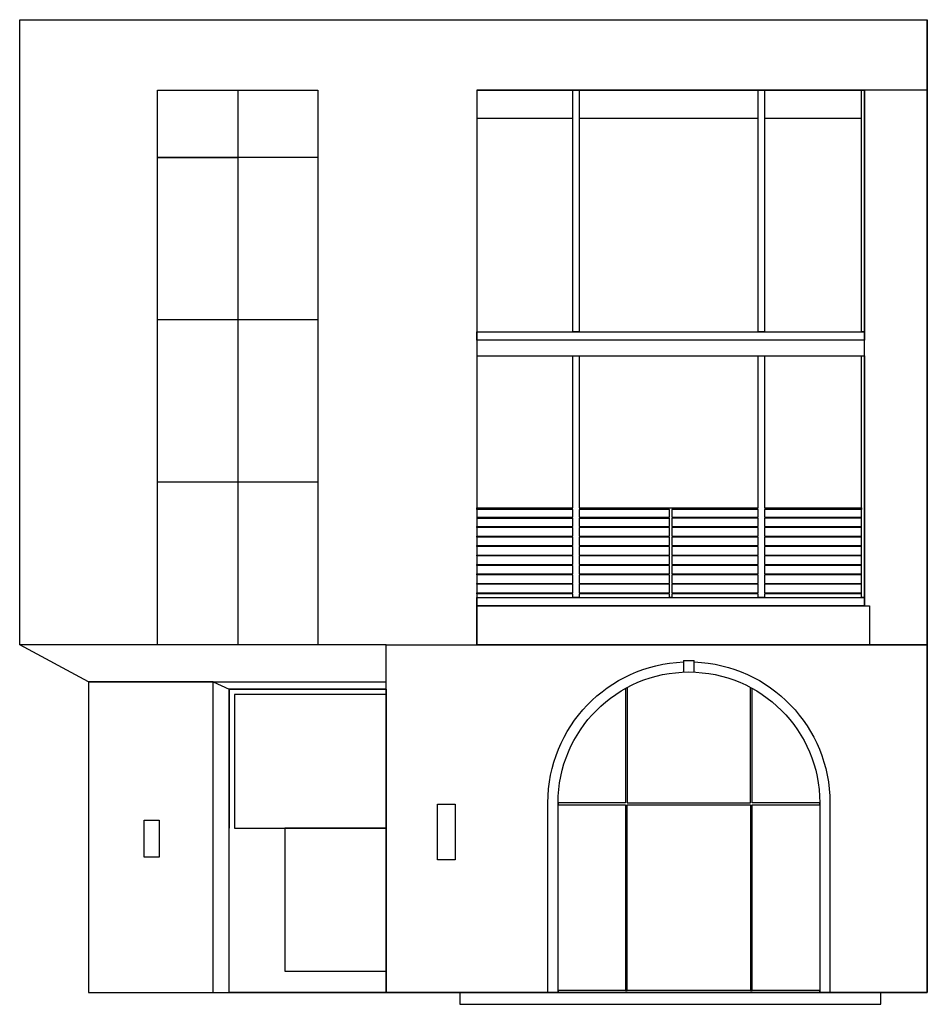
# Model space of a CAD drawing. Units: feet. Extents: x 2368 to 3224, y 836 to 1229.
# Tile 9 of 9: x 2873 to 3224, y 849 to 1229. Entities that reach past the tile are written whole.
import ezdxf

# ---------------------------------------------------------------- set-up
doc = ezdxf.new("R2010")
doc.units = ezdxf.units.FT
doc.layers.add('A-ELEV', color=7, linetype='Continuous', lineweight=25)

msp = doc.modelspace()

# ---------------------------------------------------------------- linework, layer by layer
at = {"layer": 'A-ELEV'}
for p, q in [((2872.69, 987.86), (2872.69, 1229.35)), ((3223.55, 853.51), (3223.55, 1229.35)), ((2956.97, 1202.15), (2956.97, 987.86)), ((3049.37, 1202.15), (3199.32, 1202.15)), ((3086.5, 1191.22), (3049.37, 1191.22)), ((3158.11, 1191.22), (3088.99, 1191.22)), ((3198.12, 1191.22), (3160.6, 1191.22)), ((2987.91, 1176.09), (2926.02, 1176.09)), ((3199.32, 1105.51), (3049.37, 1105.51)), ((3049.37, 1099.51), (3199.32, 1099.51)), ((3049.37, 1037.14), (3086.5, 1037.14)), ((3049.37, 1036.77), (3086.5, 1036.77)), ((3088.99, 1037.14), (3123.88, 1037.14)), ((3088.99, 1036.77), (3123.88, 1036.77)), ((3014.41, 987.86), (2872.69, 987.86)), ((2899.3, 973.51), (2872.69, 987.86)), ((2899.3, 973.51), (3014.41, 973.51)), ((2947.43, 973.51), (2953.69, 970.69)), ((2899.3, 853.51), (3223.55, 853.51))]:
    msp.add_line(p, q, dxfattribs=at)
for points in [[(2872.69, 1229.35), (3223.55, 1229.35), (3223.55, 1202.15), (3049.37, 1202.15)], [(3223.55, 1229.35), (3223.55, 987.86), (3199.32, 987.86)], [(3049.37, 1202.15), (3049.37, 987.86)], [(3199.32, 1002.87), (3199.32, 1202.15)], [(2987.91, 1113.35), (2926.02, 1113.35), (2926.02, 1176.09), (2956.97, 1176.09)], [(2987.91, 1113.35), (2987.91, 1050.6), (2926.02, 1050.6)], [(3086.5, 1040.78), (3086.5, 1099.51), (3088.99, 1099.51), (3088.99, 1040.78)], [(3158.11, 1040.78), (3158.11, 1099.51), (3160.6, 1099.51), (3160.6, 1040.78)], [(2962.72, 987.86), (2926.02, 987.86), (2926.02, 1050.6)], [(3086.5, 1040.06), (3049.37, 1040.06), (3049.37, 1040.78), (3086.5, 1040.78)], [(3086.5, 1037.14), (3086.5, 1040.06)], [(3088.99, 1040.78), (3158.11, 1040.78)], [(3088.99, 1040.06), (3088.99, 1037.14)], [(3123.88, 1040.06), (3088.99, 1040.06)], [(3123.88, 1037.14), (3123.88, 1040.06)], [(3124.82, 1040.06), (3124.82, 1037.14)], [(3158.11, 1040.06), (3124.82, 1040.06)], [(3158.11, 1037.14), (3158.11, 1040.06)], [(3160.6, 1040.78), (3198.12, 1040.78), (3198.12, 1040.06), (3160.6, 1040.06)], [(3160.6, 1040.06), (3160.6, 1037.14)], [(3086.5, 1033.48), (3086.5, 1036.77)], [(3088.99, 1036.77), (3088.99, 1033.48)], [(3123.88, 1033.48), (3123.88, 1036.77)], [(3124.82, 1037.14), (3158.11, 1037.14)], [(3124.82, 1036.77), (3124.82, 1033.48)], [(3158.11, 1036.77), (3124.82, 1036.77)], [(3158.11, 1033.48), (3158.11, 1036.77)], [(3160.6, 1037.14), (3198.12, 1037.14)], [(3198.12, 1036.77), (3160.6, 1036.77)], [(3160.6, 1036.77), (3160.6, 1033.48)], [(3199.32, 1037.14), (3199.32, 1036.77)], [(3086.5, 1033.11), (3049.37, 1033.11), (3049.37, 1033.48), (3086.5, 1033.48)], [(3086.5, 1029.83), (3086.5, 1033.11)], [(3088.99, 1033.48), (3123.88, 1033.48)], [(3088.99, 1033.11), (3088.99, 1029.83)], [(3123.88, 1033.11), (3088.99, 1033.11)], [(3123.88, 1029.83), (3123.88, 1033.11)], [(3124.82, 1033.48), (3158.11, 1033.48)], [(3124.82, 1033.11), (3124.82, 1029.83)], [(3158.11, 1033.11), (3124.82, 1033.11)], [(3158.11, 1029.83), (3158.11, 1033.11)], [(3160.6, 1033.48), (3198.12, 1033.48)], [(3198.12, 1033.11), (3160.6, 1033.11)], [(3160.6, 1033.11), (3160.6, 1029.83)], [(3199.32, 1033.48), (3199.32, 1033.11)], [(3086.5, 1029.46), (3049.37, 1029.46), (3049.37, 1029.83), (3086.5, 1029.83)], [(3086.5, 1026.18), (3086.5, 1029.46)], [(3088.99, 1029.83), (3123.88, 1029.83)], [(3088.99, 1029.46), (3088.99, 1026.18)], [(3123.88, 1029.46), (3088.99, 1029.46)], [(3123.88, 1026.18), (3123.88, 1029.46)], [(3124.82, 1029.83), (3158.11, 1029.83)], [(3124.82, 1029.46), (3124.82, 1026.18)], [(3158.11, 1029.46), (3124.82, 1029.46)], [(3158.11, 1026.18), (3158.11, 1029.46)], [(3160.6, 1029.83), (3198.12, 1029.83)], [(3198.12, 1029.46), (3160.6, 1029.46)], [(3160.6, 1029.46), (3160.6, 1026.18)], [(3199.32, 1029.83), (3199.32, 1029.46)], [(3086.5, 1025.81), (3049.37, 1025.81), (3049.37, 1026.18), (3086.5, 1026.18)], [(3086.5, 1022.52), (3086.5, 1025.81)], [(3088.99, 1026.18), (3123.88, 1026.18)], [(3088.99, 1025.81), (3088.99, 1022.52)], [(3123.88, 1025.81), (3088.99, 1025.81)], [(3123.88, 1022.52), (3123.88, 1025.81)], [(3124.82, 1026.18), (3158.11, 1026.18)], [(3124.82, 1025.81), (3124.82, 1022.52)], [(3158.11, 1025.81), (3124.82, 1025.81)], [(3158.11, 1022.52), (3158.11, 1025.81)], [(3160.6, 1026.18), (3198.12, 1026.18)], [(3198.12, 1025.81), (3160.6, 1025.81)], [(3160.6, 1025.81), (3160.6, 1022.52)], [(3199.32, 1026.18), (3199.32, 1025.81)], [(3086.5, 1022.15), (3049.37, 1022.15), (3049.37, 1022.52), (3086.5, 1022.52)], [(3086.5, 1018.87), (3086.5, 1022.15)], [(3088.99, 1022.52), (3123.88, 1022.52)], [(3088.99, 1022.15), (3088.99, 1018.87)], [(3123.88, 1022.15), (3088.99, 1022.15)], [(3123.88, 1018.87), (3123.88, 1022.15)], [(3124.82, 1022.52), (3158.11, 1022.52)], [(3124.82, 1022.15), (3124.82, 1018.87)], [(3158.11, 1022.15), (3124.82, 1022.15)], [(3158.11, 1018.87), (3158.11, 1022.15)], [(3160.6, 1022.52), (3198.12, 1022.52)], [(3198.12, 1022.15), (3160.6, 1022.15)], [(3160.6, 1022.15), (3160.6, 1018.87)], [(3199.32, 1022.52), (3199.32, 1022.15)], [(3086.5, 1018.5), (3049.37, 1018.5), (3049.37, 1018.87), (3086.5, 1018.87)], [(3086.5, 1015.21), (3086.5, 1018.5)], [(3088.99, 1018.87), (3123.88, 1018.87)], [(3088.99, 1018.5), (3088.99, 1015.21)], [(3123.88, 1018.5), (3088.99, 1018.5)], [(3123.88, 1015.21), (3123.88, 1018.5)], [(3124.82, 1018.87), (3158.11, 1018.87)], [(3124.82, 1018.5), (3124.82, 1015.21)], [(3158.11, 1018.5), (3124.82, 1018.5)], [(3158.11, 1015.21), (3158.11, 1018.5)], [(3160.6, 1018.87), (3198.12, 1018.87)], [(3198.12, 1018.5), (3160.6, 1018.5)], [(3160.6, 1018.5), (3160.6, 1015.21)], [(3199.32, 1018.87), (3199.32, 1018.5)], [(3086.5, 1014.84), (3049.37, 1014.84), (3049.37, 1015.21), (3086.5, 1015.21)], [(3086.5, 1011.56), (3086.5, 1014.84)], [(3088.99, 1015.21), (3123.88, 1015.21)], [(3088.99, 1014.84), (3088.99, 1011.56)], [(3123.88, 1014.84), (3088.99, 1014.84)], [(3123.88, 1011.56), (3123.88, 1014.84)], [(3124.82, 1015.21), (3158.11, 1015.21)], [(3124.82, 1014.84), (3124.82, 1011.56)], [(3158.11, 1014.84), (3124.82, 1014.84)], [(3158.11, 1011.56), (3158.11, 1014.84)], [(3160.6, 1015.21), (3198.12, 1015.21)], [(3198.12, 1014.84), (3160.6, 1014.84)], [(3160.6, 1014.84), (3160.6, 1011.56)], [(3199.32, 1015.21), (3199.32, 1014.84)], [(3086.5, 1011.19), (3049.37, 1011.19), (3049.37, 1011.56), (3086.5, 1011.56)], [(3086.5, 1007.9), (3086.5, 1011.19)], [(3088.99, 1011.56), (3123.88, 1011.56)], [(3088.99, 1011.19), (3088.99, 1007.9)], [(3123.88, 1011.19), (3088.99, 1011.19)], [(3123.88, 1007.9), (3123.88, 1011.19)], [(3124.82, 1011.56), (3158.11, 1011.56)], [(3124.82, 1011.19), (3124.82, 1007.9)], [(3158.11, 1011.19), (3124.82, 1011.19)], [(3158.11, 1007.9), (3158.11, 1011.19)], [(3160.6, 1011.56), (3198.12, 1011.56)], [(3198.12, 1011.19), (3160.6, 1011.19)], [(3160.6, 1011.19), (3160.6, 1007.9)], [(3199.32, 1011.56), (3199.32, 1011.19)], [(3086.5, 1007.53), (3049.37, 1007.53), (3049.37, 1007.9), (3086.5, 1007.9)], [(3088.99, 1007.53), (3088.99, 1006.11), (3086.5, 1006.11), (3086.5, 1007.53)], [(3088.99, 1007.9), (3123.88, 1007.9)], [(3123.88, 1007.53), (3088.99, 1007.53)], [(3124.82, 1007.53), (3124.82, 1006.11), (3123.88, 1006.11), (3123.88, 1007.53)], [(3124.82, 1007.9), (3158.11, 1007.9)], [(3158.11, 1007.53), (3124.82, 1007.53)], [(3160.6, 1007.53), (3160.6, 1006.11), (3158.11, 1006.11), (3158.11, 1007.53)], [(3160.6, 1007.9), (3198.12, 1007.9)], [(3198.12, 1007.53), (3160.6, 1007.53)], [(3199.32, 1007.9), (3199.32, 1007.53)], [(3129.31, 981.73), (3129.31, 977.28)], [(3133.48, 977.28), (3133.48, 981.73)], [(3014.41, 916.99), (3014.41, 970.69), (2953.69, 970.69), (2953.69, 916.99)], [(3106.9, 971), (3106.9, 926.73), (3080.81, 926.73), (3080.81, 926.06), (3106.9, 926.06), (3106.9, 854.24), (3107.58, 854.24), (3107.58, 926.06), (3155.21, 926.06), (3155.21, 854.24), (3155.89, 854.24), (3155.89, 926.06), (3181.99, 926.06), (3181.99, 926.73), (3155.89, 926.73), (3155.89, 971)], [(3107.58, 971.36), (3107.58, 926.73), (3155.21, 926.73), (3155.21, 971.36)], [(3014.41, 968.65), (2955.74, 968.65), (2955.74, 916.99)], [(2955.74, 916.99), (3014.41, 916.99), (3014.41, 853.51), (2953.69, 853.51), (2953.69, 916.99)], [(2955.74, 916.99), (2986.52, 916.99)]]:
    msp.add_lwpolyline(points, dxfattribs=at)
for points in [[(2987.91, 987.86), (2926.02, 987.86), (2926.02, 1202.15), (2987.91, 1202.15)], [(3086.5, 1202.15), (3088.99, 1202.15), (3088.99, 1108.75), (3086.5, 1108.75)], [(3158.11, 1202.15), (3160.6, 1202.15), (3160.6, 1108.75), (3158.11, 1108.75)], [(3199.32, 1108.75), (3198.12, 1108.75), (3198.12, 1202.15), (3199.32, 1202.15)], [(3199.32, 1105.51), (3049.37, 1105.51), (3049.37, 1108.75), (3199.32, 1108.75)], [(3199.32, 1006.11), (3198.12, 1006.11), (3198.12, 1099.51), (3199.32, 1099.51)], [(3199.32, 1002.87), (3049.37, 1002.87), (3049.37, 1006.11), (3199.32, 1006.11)], [(3049.37, 1002.87), (3201.24, 1002.87), (3201.24, 987.86), (3049.37, 987.86)], [(3223.55, 853.51), (3014.41, 853.51), (3014.41, 987.86), (3223.55, 987.86)], [(2899.3, 853.51), (2947.43, 853.51), (2947.43, 973.51), (2899.3, 973.51)], [(2953.69, 970.69), (3014.41, 970.69), (3014.41, 853.51), (2953.69, 853.51)], [(3034.26, 926.19), (3041.09, 926.19), (3041.09, 904.71), (3034.26, 904.71)], [(2920.79, 920.11), (2926.6, 920.11), (2926.6, 905.78), (2920.79, 905.78)], [(3014.41, 916.99), (2975.19, 916.99), (2975.19, 861.76), (3014.41, 861.76)], [(3205.53, 853.51), (3042.9, 853.51), (3042.9, 848.93), (3205.53, 848.93)], [(3080.81, 853.51), (3181.99, 853.51), (3181.99, 854.24), (3080.81, 854.24)]]:
    msp.add_lwpolyline(points, close=True, dxfattribs=at)
for points in [[(3129.31, 981.73, -0.018787), (3133.48, 981.73)], [(3076.87, 853.51), (3076.87, 926.73, -0.403049), (3129.31, 981.22, -0.403049)], [(3133.48, 981.22, -0.403049), (3185.92, 926.73), (3185.92, 853.51)], [(3080.81, 853.51), (3080.81, 926.73, -1), (3181.99, 926.73), (3181.99, 853.51)]]:
    msp.add_lwpolyline(points, format="xyb", dxfattribs=at)

doc.saveas('drawing.dxf')
